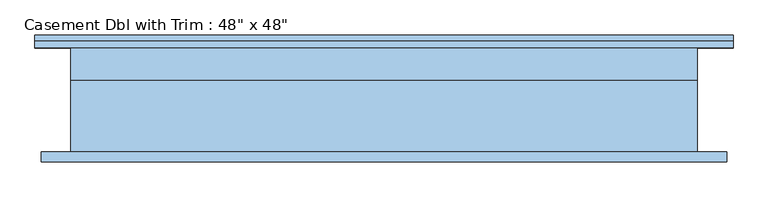
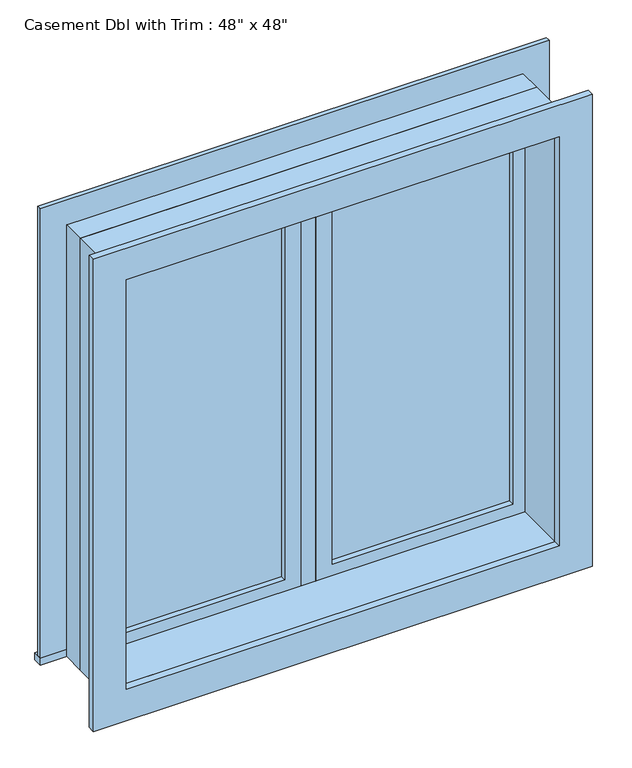
"""IFC4 building model written with IfcOpenShell, lengths in millimetres: window geometry."""

from ifc_helpers import new_model, si_unit, frame, origin, place, context, project, spatial, polyline, outline, extrude, source, transform, mapped, element, save


def window_0862ab64(model_context):
    return source(origin(), model_context, "Body", "SweptSolid", [
        extrude(outline(polyline([(63.5, 85.725), (546.1, 85.725), (546.1, 73.025), (63.5, 73.025), (63.5, 85.725)])), frame((0.0, 0.0, 977.9), z_axis=(0.0, 0.0, 1.0), x_axis=(1.0, 0.0, 0.0)), (0.0, 0.0, 1.0), 1092.2),
        extrude(outline(polyline([(2114.55, 19.05), (933.45, 19.05), (933.45, 590.55), (2114.55, 590.55), (2114.55, 19.05)]), holes=[polyline([(2070.1, 63.5), (2070.1, 546.1), (977.9, 546.1), (977.9, 63.5), (2070.1, 63.5)])]), frame((0.0, 57.15, 0.0), z_axis=(0.0, 1.0, 0.0), x_axis=(0.0, 0.0, 1.0)), (0.0, 0.0, 1.0), 44.45),
        extrude(outline(polyline([(19.05, 57.15), (-19.05, 57.15), (-19.05, 120.65), (19.05, 120.65), (19.05, 57.15)])), frame((0.0, 0.0, 933.45), z_axis=(0.0, 0.0, 1.0), x_axis=(1.0, 0.0, 0.0)), (0.0, 0.0, 1.0), 1181.1),
        extrude(outline(polyline([(-679.45, 146.05), (679.45, 146.05), (679.45, 120.65), (-679.45, 120.65), (-679.45, 146.05)])), frame((0.0, 0.0, 914.4), z_axis=(0.0, 0.0, 1.0), x_axis=(1.0, 0.0, 0.0)), (0.0, 0.0, 1.0), 19.05),
        extrude(outline(polyline([(2114.55, -590.55), (2114.55, 590.55), (933.45, 590.55), (933.45, 679.45), (2203.45, 679.45), (2203.45, -679.45), (933.45, -679.45), (933.45, -590.55), (2114.55, -590.55)])), frame((0.0, 120.65, 0.0), z_axis=(0.0, 1.0, 0.0), x_axis=(0.0, 0.0, 1.0)), (0.0, 0.0, 1.0), 12.7),
        extrude(outline(polyline([(2190.75, 666.75), (2190.75, -666.75), (857.25, -666.75), (857.25, 666.75), (2190.75, 666.75)]), holes=[polyline([(2101.85, 577.85), (946.15, 577.85), (946.15, -577.85), (2101.85, -577.85), (2101.85, 577.85)])]), frame((0.0, -101.6, 0.0), z_axis=(0.0, 1.0, 0.0), x_axis=(0.0, 0.0, 1.0)), (0.0, 0.0, 1.0), 19.05),
        extrude(outline(polyline([(-63.5, 73.025), (-546.1, 73.025), (-546.1, 85.725), (-63.5, 85.725), (-63.5, 73.025)])), frame((0.0, 0.0, 977.9), z_axis=(0.0, 0.0, 1.0), x_axis=(1.0, 0.0, 0.0)), (0.0, 0.0, 1.0), 1092.2),
        extrude(outline(polyline([(2114.55, -590.55), (933.45, -590.55), (933.45, -19.05), (2114.55, -19.05), (2114.55, -590.55)]), holes=[polyline([(2070.1, -546.1), (2070.1, -63.5), (977.9, -63.5), (977.9, -546.1), (2070.1, -546.1)])]), frame((0.0, 57.15, 0.0), z_axis=(0.0, 1.0, 0.0), x_axis=(0.0, 0.0, 1.0)), (0.0, 0.0, 1.0), 44.45),
        extrude(outline(polyline([(2133.6, -609.6), (914.4, -609.6), (914.4, 609.6), (2133.6, 609.6), (2133.6, -609.6)]), holes=[polyline([(2101.85, -577.85), (2101.85, 577.85), (946.15, 577.85), (946.15, -577.85), (2101.85, -577.85)])]), frame((0.0, -82.55, 0.0), z_axis=(0.0, 1.0, 0.0), x_axis=(0.0, 0.0, 1.0)), (0.0, 0.0, 1.0), 139.7),
        extrude(outline(polyline([(2133.6, 609.6), (2133.6, -609.6), (914.4, -609.6), (914.4, 609.6), (2133.6, 609.6)]), holes=[polyline([(2114.55, 590.55), (933.45, 590.55), (933.45, -590.55), (2114.55, -590.55), (2114.55, 590.55)])]), frame((0.0, 57.15, 0.0), z_axis=(0.0, 1.0, 0.0), x_axis=(0.0, 0.0, 1.0)), (0.0, 0.0, 1.0), 63.5),
    ])


if __name__ == "__main__":
    model = new_model("IFC4")
    model_context = context("Model", 3, world=origin())
    ifc_project = project(units=[si_unit("LENGTHUNIT", "METRE", prefix="MILLI")], contexts=[model_context])
    site = spatial("IfcSite", under=ifc_project)
    building = spatial("IfcBuilding", under=site)
    placement = place(None, origin())
    window_shape = window_0862ab64(model_context)
    element("IfcWindow", 1, ObjectType="Casement Dbl with Trim : 48\" x 48\"", at=placement, inside=building, context=model_context, shape_type="MappedRepresentation", body=[
        mapped(window_shape, transform((0.0, 0.0, 0.0), x_axis=(1.0, 0.0, 0.0), y_axis=(0.0, 1.0, 0.0), z_axis=(0.0, 0.0, 1.0))),
    ])
    save(model, "model.ifc")

# Revit data of these elements
# Type "Casement Dbl with Trim : 48\" x 48\""
#   Type Mark = "10"
#   Construction Type Id = "GSP4R"
#   Assembly Code = "B2020100"
#   Analytic Construction = "1/8 in Pilkington single glazing"
#   Visual Light Transmittance = 0.9
#   Thermal Resistance (R) = 1.53941 (h·ft²·°F)/BTU
#   Solar Heat Gain Coefficient = 0.78
#   Heat Transfer Coefficient (U) = 0.6496 BTU/(h·ft²·°F)
#   Height = 4' - 0"
#   Default Sill Height = 3' - 0"
#   Trim Projection - Ext. = 0' - 0 1/2"
#   Trim Projection - Int. = 0' - 0 3/4"
#   Trim Width - Exterior = 0' - 3 1/2"
#   Trim Width - Interior = 0' - 3 1/2"
#   Width = 4' - 0"
#   Window Inset = 0' - 0 3/4"
#   Define Thermal Properties by = 1
#   Glass Pane Material = Glass
#   Sash Material = Sash
#   Trim Exterior Material = Trim
#   Trim Interior Material = Trim
#   Wall Closure = (empty or 0)
# Element 1 (IfcWindow, "Casement Dbl with Trim : 48\" x 48\"")
#   Materials on its faces: "Sash", "Trim", "Glass"
# Materials
#   "Glass": class "Glass", colour RGB 0 128 192, transparency 0.75, Description = "Soda Lime Glass", Cost = 0
#   "Sash": class "Wood", colour RGB 224 178 126, transparency 0
#   "Trim": class "Wood", colour RGB 224 178 126, transparency 0
